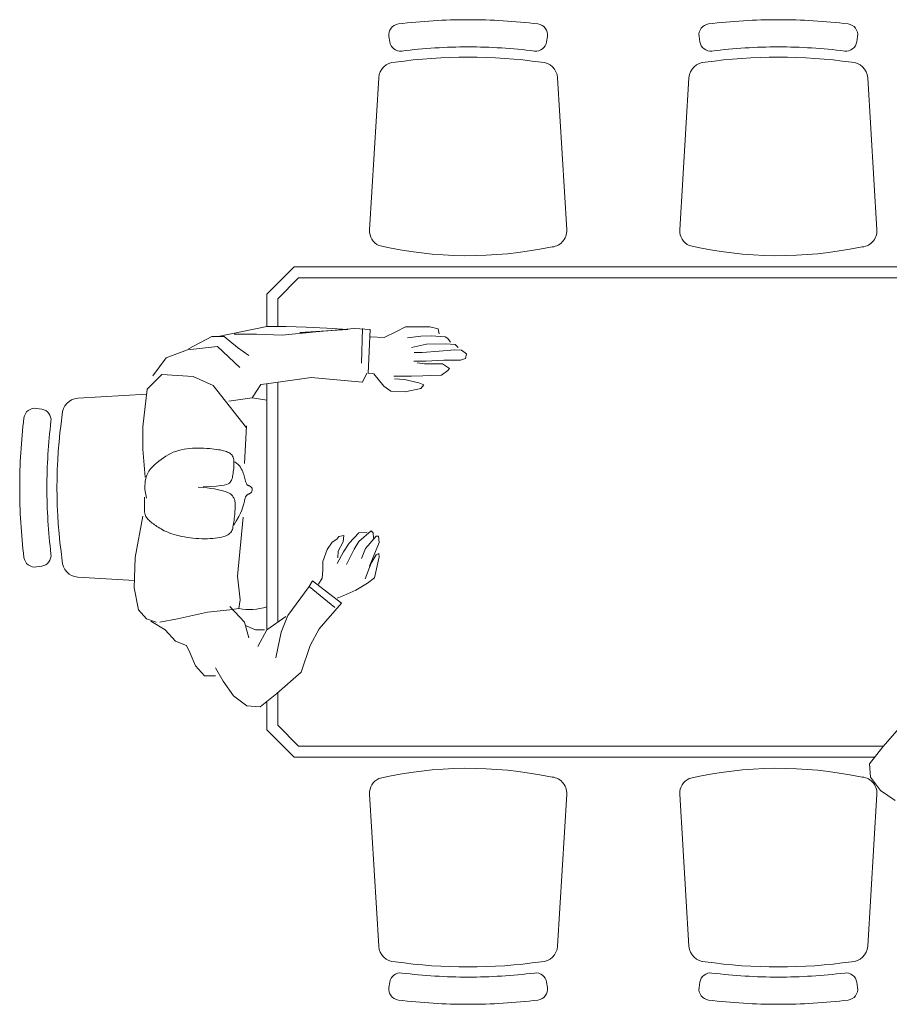
# Model space of a CAD drawing. Units: inches. Extents: x 1913 to 5309, y 1003 to 1733.
# Tile 5 of 23: x 2200 to 2248, y 1415 to 1469. Entities that reach past the tile are written whole.
import ezdxf

# ---------------------------------------------------------------- set-up
doc = ezdxf.new("R2010")
doc.units = ezdxf.units.IN
doc.layers.add('A-FURN', color=8, linetype='Continuous', lineweight=18)

# ---------------------------------------------------------------- blocks, each defined once
blk = doc.blocks.new('A$C421907B3')
for p, q in [((0.7245, 2.5796), (0.7652, 2.5876)), ((0.7652, 2.5876), (0.8209, 2.5856)), ((0.7079, 2.565), (0.7245, 2.5796)), ((0.8209, 2.5856), (0.8965, 2.5714)), ((0.9043, 2.5682), (0.9018, 2.5678)), ((0.9071, 2.5684), (0.9043, 2.5682)), ((0.9102, 2.5686), (0.9071, 2.5684)), ((0.9137, 2.5687), (0.9102, 2.5686)), ((0.9175, 2.5687), (0.9137, 2.5687)), ((0.9217, 2.5687), (0.9175, 2.5687)), ((0.9264, 2.5687), (0.9217, 2.5687)), ((0.9314, 2.5687), (0.9264, 2.5687)), ((0.9684, 2.5672), (1.0195, 2.5715)), ((1.0195, 2.5715), (1.0607, 2.5715)), ((1.0607, 2.5715), (1.1301, 2.5633)), ((0.7038, 2.5568), (0.6875, 2.5302)), ((0.7017, 2.5468), (0.7079, 2.565)), ((0.8808, 2.55), (0.8792, 2.5478)), ((0.8823, 2.5521), (0.8808, 2.55)), ((0.8839, 2.5541), (0.8823, 2.5521)), ((0.8853, 2.556), (0.8839, 2.5541)), ((0.8868, 2.5577), (0.8853, 2.556)), ((0.8883, 2.5594), (0.8868, 2.5577)), ((0.8897, 2.5609), (0.8883, 2.5594)), ((0.8911, 2.5623), (0.8897, 2.5609)), ((0.8926, 2.5635), (0.8911, 2.5623)), ((0.8941, 2.5647), (0.8926, 2.5635)), ((0.8958, 2.5657), (0.8941, 2.5647)), ((0.8976, 2.5665), (0.8958, 2.5657)), ((0.8996, 2.5672), (0.8976, 2.5665)), ((0.9018, 2.5678), (0.8996, 2.5672)), ((0.9361, 2.5662), (0.9297, 2.5647)), ((0.942, 2.5671), (0.9361, 2.5662)), ((0.9475, 2.5676), (0.942, 2.5671)), ((0.9525, 2.5677), (0.9475, 2.5676)), ((0.9571, 2.5675), (0.9525, 2.5677)), ((0.9614, 2.5669), (0.9571, 2.5675)), ((0.9652, 2.5662), (0.9614, 2.5669)), ((0.9686, 2.5653), (0.9652, 2.5662)), ((0.9717, 2.5643), (0.9686, 2.5653)), ((0.9745, 2.5632), (0.9717, 2.5643)), ((0.977, 2.5619), (0.9745, 2.5632)), ((0.9794, 2.5605), (0.977, 2.5619)), ((0.9818, 2.5588), (0.9794, 2.5605)), ((0.9841, 2.5568), (0.9818, 2.5588)), ((0.9865, 2.5545), (0.9841, 2.5568)), ((0.9891, 2.5519), (0.9865, 2.5545)), ((0.9918, 2.5489), (0.9891, 2.5519)), ((1.1301, 2.5633), (1.1567, 2.5368)), ((1.1546, 2.5531), (1.1875, 2.5285)), ((0.7017, 2.5405), (0.7079, 2.5077)), ((0.8699, 2.5321), (0.8684, 2.5289)), ((0.8714, 2.5351), (0.8699, 2.5321)), ((0.873, 2.5379), (0.8714, 2.5351)), ((0.8745, 2.5405), (0.873, 2.5379)), ((0.8761, 2.543), (0.8745, 2.5405)), ((0.8777, 2.5455), (0.8761, 2.543)), ((0.8792, 2.5478), (0.8777, 2.5455)), ((0.9948, 2.5455), (0.9918, 2.5489)), ((0.9978, 2.5419), (0.9948, 2.5455)), ((1.0008, 2.5379), (0.9978, 2.5419)), ((1.0037, 2.5338), (1.0008, 2.5379)), ((1.0066, 2.5294), (1.0037, 2.5338)), ((1.1567, 2.5368), (1.153, 2.4792)), ((0.6875, 2.5302), (0.6672, 2.5117)), ((0.8628, 2.514), (0.8616, 2.5096)), ((0.8641, 2.5181), (0.8628, 2.514)), ((0.8655, 2.522), (0.8641, 2.5181)), ((0.8669, 2.5256), (0.8655, 2.522)), ((0.8684, 2.5289), (0.8669, 2.5256)), ((1.0093, 2.5249), (1.0066, 2.5294)), ((1.0117, 2.5203), (1.0093, 2.5249)), ((1.0138, 2.5155), (1.0117, 2.5203)), ((1.0156, 2.5107), (1.0138, 2.5155)), ((1.1875, 2.5285), (1.202, 2.4895)), ((0.6672, 2.5117), (0.6589, 2.4912)), ((0.7079, 2.5077), (0.7204, 2.4524)), ((0.8594, 2.5001), (0.8584, 2.4951)), ((0.8604, 2.5049), (0.8594, 2.5001)), ((0.8616, 2.5096), (0.8604, 2.5049)), ((1.0171, 2.5058), (1.0156, 2.5107)), ((1.0184, 2.5008), (1.0171, 2.5058)), ((1.0194, 2.4958), (1.0184, 2.5008)), ((1.0202, 2.4907), (1.0194, 2.4958)), ((0.6464, 2.4852), (0.6219, 2.4749)), ((0.6589, 2.4912), (0.6464, 2.4852)), ((0.8562, 2.4794), (0.8558, 2.474)), ((0.8568, 2.4847), (0.8562, 2.4794)), ((0.8576, 2.49), (0.8568, 2.4847)), ((0.8584, 2.4951), (0.8576, 2.49)), ((1.0208, 2.4855), (1.0202, 2.4907)), ((1.0212, 2.4802), (1.0208, 2.4855)), ((1.0214, 2.4749), (1.0212, 2.4802)), ((1.153, 2.4792), (1.1364, 2.4424)), ((1.202, 2.4895), (1.2083, 2.4342)), ((1.2041, 2.4875), (1.2266, 2.4445)), ((0.6219, 2.4749), (0.6036, 2.4584)), ((0.8552, 2.4632), (0.8551, 2.4579)), ((0.8554, 2.4686), (0.8552, 2.4632)), ((0.8558, 2.474), (0.8554, 2.4686)), ((0.9483, 2.453), (0.9491, 2.4609)), ((0.9491, 2.4609), (0.9498, 2.4698)), ((0.9505, 2.4603), (0.9511, 2.447)), ((1.0212, 2.4591), (1.0214, 2.4643)), ((1.0215, 2.4696), (1.0214, 2.4749)), ((1.0214, 2.4643), (1.0215, 2.4696)), ((0.6036, 2.4584), (0.6036, 2.4379)), ((0.7204, 2.4524), (0.7246, 2.4114)), ((0.8551, 2.4579), (0.8552, 2.4527)), ((0.8552, 2.4527), (0.8554, 2.4476)), ((0.8554, 2.4476), (0.8557, 2.4428)), ((0.8557, 2.4428), (0.8561, 2.4383)), ((0.9465, 2.4399), (0.9474, 2.446)), ((0.9474, 2.446), (0.9483, 2.453)), ((0.9511, 2.447), (0.9518, 2.4364)), ((1.0197, 2.4402), (1.0202, 2.4445)), ((1.0202, 2.4445), (1.0206, 2.4492)), ((1.0206, 2.4492), (1.021, 2.4541)), ((1.021, 2.4541), (1.0212, 2.4591)), ((1.1364, 2.4424), (1.0587, 2.3808)), ((1.2266, 2.4445), (1.2266, 2.422)), ((0.5933, 2.4236), (0.5667, 2.4051)), ((0.6178, 2.4379), (0.5933, 2.4236)), ((0.8561, 2.4383), (0.8567, 2.4341)), ((0.8567, 2.4341), (0.8574, 2.4301)), ((0.8574, 2.4301), (0.8582, 2.4265)), ((0.8582, 2.4265), (0.8591, 2.4232)), ((0.9425, 2.4226), (0.9435, 2.426)), ((0.9435, 2.426), (0.9445, 2.43)), ((0.9445, 2.43), (0.9455, 2.4346)), ((0.9455, 2.4346), (0.9465, 2.4399)), ((0.9518, 2.4364), (0.9526, 2.4283)), ((0.9526, 2.4283), (0.9535, 2.4222)), ((1.0168, 2.423), (1.0174, 2.4259)), ((1.0174, 2.4259), (1.0181, 2.429)), ((1.0181, 2.429), (1.0186, 2.4325)), ((1.0186, 2.4325), (1.0192, 2.4362)), ((1.0192, 2.4362), (1.0197, 2.4402)), ((1.2083, 2.4342), (1.1693, 2.3932)), ((1.2447, 2.3435), (1.2266, 2.4332)), ((0.7308, 2.4114), (0.7018, 2.3846)), ((0.7246, 2.4114), (0.7267, 2.3949)), ((0.8591, 2.4232), (0.8601, 2.4202)), ((0.8601, 2.4202), (0.8612, 2.4176)), ((0.8612, 2.4176), (0.8624, 2.4152)), ((0.8624, 2.4152), (0.8637, 2.4132)), ((0.8637, 2.4132), (0.8651, 2.4114)), ((0.8651, 2.4114), (0.8666, 2.41)), ((0.8666, 2.41), (0.8682, 2.4088)), ((0.8682, 2.4088), (0.87, 2.4078)), ((0.87, 2.4078), (0.872, 2.407)), ((0.872, 2.407), (0.8742, 2.4063)), ((0.8742, 2.4063), (0.8767, 2.4058)), ((0.8767, 2.4058), (0.8794, 2.4052)), ((0.8794, 2.4052), (0.8824, 2.4048)), ((0.9315, 2.4052), (0.9329, 2.406)), ((0.9329, 2.406), (0.9341, 2.4069)), ((0.9341, 2.4069), (0.9353, 2.4079)), ((0.9353, 2.4079), (0.9363, 2.409)), ((0.9363, 2.409), (0.9373, 2.4102)), ((0.9373, 2.4102), (0.9382, 2.4116)), ((0.9382, 2.4116), (0.9391, 2.4131)), ((0.9391, 2.4131), (0.9399, 2.415)), ((0.9399, 2.415), (0.9408, 2.4171)), ((0.9408, 2.4171), (0.9416, 2.4196)), ((0.9416, 2.4196), (0.9425, 2.4226)), ((0.9535, 2.4222), (0.9546, 2.4177)), ((0.9546, 2.4177), (0.9558, 2.4146)), ((0.9558, 2.4146), (0.9572, 2.4124)), ((0.9572, 2.4124), (0.9588, 2.4109)), ((0.9588, 2.4109), (0.9606, 2.4096)), ((0.9606, 2.4096), (0.9626, 2.4086)), ((0.9626, 2.4086), (0.9647, 2.4077)), ((0.9647, 2.4077), (0.9671, 2.407)), ((0.9671, 2.407), (0.9696, 2.4064)), ((0.9696, 2.4064), (0.9722, 2.406)), ((0.9722, 2.406), (0.9751, 2.4055)), ((0.9751, 2.4055), (0.9781, 2.4052)), ((0.9781, 2.4052), (0.9812, 2.4048)), ((1.0025, 2.4049), (1.0047, 2.4055)), ((1.0047, 2.4055), (1.0067, 2.4064)), ((1.0067, 2.4064), (1.0085, 2.4075)), ((1.0085, 2.4075), (1.01, 2.4087)), ((1.01, 2.4087), (1.0113, 2.4102)), ((1.0113, 2.4102), (1.0124, 2.4119)), ((1.0124, 2.4119), (1.0135, 2.4137)), ((1.0135, 2.4137), (1.0144, 2.4158)), ((1.0144, 2.4158), (1.0152, 2.418)), ((1.0152, 2.418), (1.016, 2.4204)), ((1.016, 2.4204), (1.0168, 2.423)), ((1.1077, 2.4136), (1.114, 2.3706)), ((1.2266, 2.422), (1.2062, 2.3974)), ((0.5667, 2.4051), (0.5484, 2.3805)), ((0.7267, 2.3949), (0.7429, 2.3929)), ((0.7429, 2.3929), (0.7861, 2.3972)), ((0.7861, 2.3972), (0.8946, 2.387)), ((0.8801, 2.4042), (0.8884, 2.3992)), ((0.8824, 2.4048), (0.8857, 2.4043)), ((0.8857, 2.4043), (0.8891, 2.4039)), ((0.8884, 2.3992), (0.8957, 2.3952)), ((0.8891, 2.4039), (0.8925, 2.4035)), ((0.8925, 2.4035), (0.896, 2.4031)), ((0.8957, 2.3952), (0.9019, 2.3921)), ((0.896, 2.4031), (0.8995, 2.4027)), ((0.8995, 2.4027), (0.9028, 2.4024)), ((0.9019, 2.3921), (0.9073, 2.3897)), ((0.9028, 2.4024), (0.9059, 2.4022)), ((0.9059, 2.4022), (0.9088, 2.4019)), ((0.9073, 2.3897), (0.9119, 2.3881)), ((0.9088, 2.4019), (0.9114, 2.4018)), ((0.9114, 2.4018), (0.9138, 2.4016)), ((0.9119, 2.3881), (0.9157, 2.3869)), ((0.9138, 2.4016), (0.9161, 2.4016)), ((0.9161, 2.4016), (0.9182, 2.4016)), ((0.9182, 2.4016), (0.9201, 2.4017)), ((0.9201, 2.4017), (0.9219, 2.4019)), ((0.9219, 2.4019), (0.9237, 2.4022)), ((0.9237, 2.4022), (0.9254, 2.4026)), ((0.9254, 2.4026), (0.927, 2.4031)), ((0.927, 2.4031), (0.9286, 2.4037)), ((0.9286, 2.4037), (0.9301, 2.4044)), ((0.9301, 2.4044), (0.9315, 2.4052)), ((0.9757, 2.387), (0.9784, 2.388)), ((0.9784, 2.388), (0.9811, 2.3892)), ((0.9811, 2.3892), (0.9837, 2.3905)), ((0.9812, 2.4048), (0.9844, 2.4045)), ((0.9837, 2.3905), (0.9863, 2.3922)), ((0.9844, 2.4045), (0.9877, 2.4043)), ((0.9863, 2.3922), (0.9889, 2.3941)), ((0.9877, 2.4043), (0.9909, 2.4041)), ((0.9889, 2.3941), (0.9915, 2.3965)), ((0.9909, 2.4041), (0.9941, 2.4041)), ((0.9915, 2.3965), (0.994, 2.3993)), ((0.994, 2.3993), (0.9965, 2.4026)), ((0.9941, 2.4041), (0.9971, 2.4042)), ((0.9971, 2.4042), (0.9999, 2.4044)), ((0.9999, 2.4044), (1.0025, 2.4049)), ((1.2062, 2.3974), (1.1917, 2.3769)), ((1.2308, 2.3624), (1.2308, 2.4035)), ((0.5484, 2.3805), (0.5463, 2.356)), ((0.7018, 2.3846), (0.6731, 2.3766)), ((0.6876, 2.3643), (0.6959, 2.3826)), ((0.9157, 2.3869), (0.919, 2.386)), ((0.919, 2.386), (0.9217, 2.3854)), ((0.9217, 2.3854), (0.924, 2.3849)), ((0.924, 2.3849), (0.926, 2.3844)), ((0.926, 2.3844), (0.9277, 2.384)), ((0.9277, 2.384), (0.929, 2.3837)), ((0.929, 2.3837), (0.9302, 2.3833)), ((0.9302, 2.3833), (0.9312, 2.383)), ((0.9312, 2.383), (0.932, 2.3826)), ((0.932, 2.3826), (0.9327, 2.3823)), ((0.9327, 2.3823), (0.9334, 2.3818)), ((0.9334, 2.3818), (0.934, 2.3813)), ((0.934, 2.3813), (0.9346, 2.3808)), ((0.9346, 2.3808), (0.9351, 2.3803)), ((0.9351, 2.3803), (0.9356, 2.3797)), ((0.9356, 2.3797), (0.936, 2.379)), ((0.936, 2.379), (0.9365, 2.3783)), ((0.9365, 2.3783), (0.9369, 2.3776)), ((0.9369, 2.3776), (0.9372, 2.3769)), ((0.9372, 2.3769), (0.9376, 2.3761)), ((0.9376, 2.3761), (0.938, 2.3753)), ((0.938, 2.3753), (0.9384, 2.3746)), ((0.9384, 2.3746), (0.9389, 2.3738)), ((0.9389, 2.3738), (0.9395, 2.3731)), ((0.9395, 2.3731), (0.9401, 2.3725)), ((0.9401, 2.3725), (0.9408, 2.3719)), ((0.9408, 2.3719), (0.9417, 2.3714)), ((0.9417, 2.3714), (0.9426, 2.371)), ((0.9426, 2.371), (0.9437, 2.3707)), ((0.9437, 2.3707), (0.9447, 2.3706)), ((0.9447, 2.3706), (0.9458, 2.3705)), ((0.9458, 2.3705), (0.9468, 2.3706)), ((0.9468, 2.3706), (0.9478, 2.3708)), ((0.9478, 2.3708), (0.9487, 2.3712)), ((0.9487, 2.3712), (0.9494, 2.3717)), ((0.9494, 2.3717), (0.9501, 2.3723)), ((0.9501, 2.3723), (0.9507, 2.3731)), ((0.9507, 2.3731), (0.9512, 2.3739)), ((0.9512, 2.3739), (0.9517, 2.3747)), ((0.9517, 2.3747), (0.9521, 2.3755)), ((0.9521, 2.3755), (0.9524, 2.3764)), ((0.9524, 2.3764), (0.9527, 2.3771)), ((0.9527, 2.3771), (0.953, 2.3778)), ((0.953, 2.3778), (0.9533, 2.3785)), ((0.9533, 2.3785), (0.9536, 2.379)), ((0.9536, 2.379), (0.954, 2.3796)), ((0.954, 2.3796), (0.9546, 2.3801)), ((0.9546, 2.3801), (0.9554, 2.3805)), ((0.9554, 2.3805), (0.9564, 2.381)), ((0.9564, 2.381), (0.9577, 2.3815)), ((0.9577, 2.3815), (0.9593, 2.382)), ((0.9593, 2.382), (0.9611, 2.3826)), ((0.9611, 2.3826), (0.9632, 2.3832)), ((0.9632, 2.3832), (0.9655, 2.3838)), ((0.9655, 2.3838), (0.9679, 2.3845)), ((0.9679, 2.3845), (0.9705, 2.3853)), ((0.9705, 2.3853), (0.9731, 2.3861)), ((0.9731, 2.3861), (0.9757, 2.387)), ((0.9931, 2.3848), (1.0625, 2.3808)), ((1.114, 2.3706), (1.1095, 2.3436)), ((1.114, 2.3706), (1.1385, 2.3544)), ((0.5463, 2.356), (0.5709, 2.3252)), ((0.6569, 2.3601), (0.6876, 2.3438)), ((0.6876, 2.3478), (0.6876, 2.3643)), ((1.1385, 2.3544), (1.1406, 2.3358)), ((1.2287, 2.3154), (1.2308, 2.3624)), ((0.6876, 2.3438), (0.7122, 2.3088)), ((1.1406, 2.3358), (1.151, 2.262)), ((0.5709, 2.3252), (0.6099, 2.2802)), ((0.6835, 2.317), (0.6365, 2.3273)), ((0.7143, 2.3048), (0.6835, 2.317)), ((1.235, 2.2538), (1.2287, 2.3154)), ((0.7674, 2.2656), (0.7143, 2.3048)), ((0.6099, 2.2802), (0.659, 2.2637)), ((0.659, 2.2637), (0.6898, 2.2475)), ((0.7288, 2.2187), (0.7675, 2.2658)), ((0.7675, 2.2658), (0.7779, 2.2598)), ((1.151, 2.262), (1.1428, 2.1677)), ((0.6898, 2.2475), (0.7368, 2.2065)), ((0.7779, 2.2598), (0.7368, 2.2065)), ((0.7716, 2.2487), (0.7827, 2.2421)), ((1.2413, 2.1822), (1.235, 2.2538)), ((0.7827, 2.2421), (0.7969, 2.2406)), ((0.7969, 2.2406), (0.8131, 2.2406)), ((0.8131, 2.2406), (0.8354, 2.2325)), ((0.8354, 2.2325), (0.8487, 2.2236)), ((0.7509, 2.2021), (0.7458, 2.2146)), ((0.8094, 2.2146), (0.8309, 2.2028)), ((0.8324, 2.2124), (0.8198, 2.2132)), ((0.8494, 2.2036), (0.8324, 2.2124)), ((0.8487, 2.2236), (0.8546, 2.2147)), ((0.8546, 2.2147), (0.859, 2.211)), ((0.859, 2.211), (0.8613, 2.2021)), ((0.7606, 2.1798), (0.7509, 2.2021)), ((0.8079, 2.1969), (0.8361, 2.1828)), ((0.8309, 2.2028), (0.8472, 2.1925)), ((0.8472, 2.1925), (0.8658, 2.1747)), ((0.8613, 2.2021), (0.8494, 2.2036)), ((0.7732, 2.1583), (0.7606, 2.1798)), ((0.8361, 2.1828), (0.8502, 2.1747)), ((0.8502, 2.1747), (0.8695, 2.1518)), ((0.8658, 2.1747), (0.8672, 2.1591)), ((1.2392, 2.1535), (1.2413, 2.1822)), ((0.7835, 2.1457), (0.7732, 2.1583)), ((0.7814, 2.1628), (0.8102, 2.1517)), ((0.848, 2.1369), (0.805, 2.1547)), ((0.8191, 2.1695), (0.8369, 2.1621)), ((0.8369, 2.1621), (0.8599, 2.1429)), ((1.1428, 2.1677), (1.159, 2.1597)), ((1.1595, 2.1573), (1.158, 2.1467)), ((1.1595, 2.1573), (1.2392, 2.1535)), ((1.1777, 2.1697), (1.2413, 2.1677)), ((1.226, 2.1528), (1.2245, 2.1279)), ((0.8221, 2.1369), (0.7835, 2.1457)), ((0.8102, 2.1517), (0.8257, 2.1428)), ((0.828, 2.1376), (0.8221, 2.1369)), ((0.8257, 2.1428), (0.828, 2.1376)), ((0.8599, 2.1384), (0.848, 2.1369)), ((0.8658, 2.1481), (0.8561, 2.1473)), ((0.8599, 2.1429), (0.8599, 2.1384)), ((0.8695, 2.1518), (0.8658, 2.1481)), ((1.158, 2.1467), (1.1354, 2.1286)), ((1.1354, 2.1286), (1.1263, 2.1158)), ((1.2245, 2.1279), (1.2358, 2.1052)), ((1.1263, 2.1158), (1.1248, 2.0893)), ((1.1474, 2.0909), (1.149, 2.1089)), ((1.1535, 2.1105), (1.1536, 2.078)), ((1.2358, 2.1052), (1.2442, 2.0886)), ((1.1248, 2.0893), (1.1308, 2.0606)), ((1.1414, 2.0644), (1.1474, 2.0909)), ((1.2238, 2.0848), (1.2269, 2.0606)), ((1.2442, 2.0886), (1.2442, 2.0441)), ((1.1377, 2.0553), (1.1414, 2.0644)), ((1.1536, 2.078), (1.1543, 2.0568)), ((1.1762, 2.0539), (1.1784, 2.0674)), ((1.1815, 2.0735), (1.1815, 2.0516)), ((1.1974, 2.0584), (1.1974, 2.0727)), ((1.2064, 2.078), (1.2125, 2.0501)), ((1.1308, 2.0606), (1.1377, 2.0553)), ((1.1543, 2.0568), (1.1551, 2.0432)), ((1.1762, 2.0357), (1.1762, 2.0539)), ((1.1815, 2.0516), (1.1831, 2.0183)), ((1.1996, 2.0267), (1.1974, 2.0584)), ((1.2125, 2.0501), (1.2132, 2.0154)), ((1.2269, 2.0606), (1.2276, 2.0418)), ((1.2442, 2.0441), (1.2404, 2.029)), ((1.1551, 2.0432), (1.1558, 2.0229)), ((1.1762, 2.0206), (1.1762, 2.0357)), ((1.2019, 1.9979), (1.1996, 2.0267)), ((1.2276, 2.0418), (1.2261, 2.0161)), ((1.2404, 2.029), (1.2314, 2.0267)), ((1.1558, 2.0229), (1.1641, 2.0108)), ((1.1641, 2.0108), (1.168, 2.0077)), ((1.168, 2.0077), (1.1762, 2.0206)), ((1.1831, 2.0183), (1.1831, 1.9874)), ((1.2132, 2.0154), (1.2117, 1.9972)), ((1.223, 2.0108), (1.2163, 2.0063)), ((1.2261, 2.0161), (1.223, 2.0108)), ((1.2012, 1.9859), (1.2019, 1.9979)), ((1.2117, 1.9972), (1.2064, 1.9919)), ((1.1831, 1.9874), (1.186, 1.9783)), ((1.186, 1.9783), (1.1944, 1.9768)), ((1.1944, 1.9768), (1.2012, 1.9859)), ((0.3928, 1.2157), (0.4173, 1.234)), ((0.4173, 1.234), (0.4418, 1.2361)), ((0.4418, 1.2361), (0.4726, 1.2115)), ((0.3742, 1.1891), (0.3928, 1.2157)), ((0.4726, 1.2115), (0.5176, 1.1724))]:
    blk.add_line(p, q)
at = {"ltscale": 0.1}
for points in [[(0.9489, 2.7478, 0.030867), (0.827, 2.7403, -0.408428), (0.8047, 2.7573), (0.8033, 2.7672, -0.419966), (0.8206, 2.7899, -0.030916), (0.9489, 2.7978, -0.030916), (1.0772, 2.7899, -0.419966), (1.0945, 2.7672), (1.0931, 2.7573, -0.408428), (1.0708, 2.7403, 0.030867)], [(0.0782, 2.1079, -0.399285), (0.1067, 2.1378), (0.3861, 2.1548, -0.305593), (0.4148, 2.1375, -0.109362), (0.4176, 1.8225, -0.429301), (0.3861, 1.7925), (0.1067, 1.8094, -0.399285), (0.0782, 1.8394, -0.071734)], [(1.7302, 2.1079, 0.399285), (1.7017, 2.1378), (1.4223, 2.1548, 0.305593), (1.3936, 2.1375, 0.109362), (1.3908, 1.8225, 0.429301), (1.4223, 1.7925), (1.7017, 1.8094, 0.399285), (1.7302, 1.8394, 0.071734)], [(0.05, 1.9736, 0.030867), (0.0575, 1.8517, -0.408428), (0.0405, 1.8294), (0.0306, 1.828, -0.419966), (0.0079, 1.8453, -0.030916), (0, 1.9736, -0.030916), (0.0079, 2.1019, -0.419966), (0.0306, 2.1193), (0.0405, 2.1178, -0.408428), (0.0575, 2.0956, 0.030867)], [(1.7584, 1.9736, -0.030867), (1.7509, 1.8517, 0.408428), (1.7679, 1.8294), (1.7778, 1.828, 0.419966), (1.8005, 1.8453, 0.030916), (1.8084, 1.9736, 0.030916), (1.8005, 2.1019, 0.419966), (1.7778, 2.1193), (1.7679, 2.1178, 0.408428), (1.7509, 2.0956, -0.030867)], [(0.0782, 1.5378, -0.399285), (0.1067, 1.5678), (0.3861, 1.5847, -0.305593), (0.4148, 1.5674, -0.109362), (0.4176, 1.2524, -0.429301), (0.3861, 1.2224), (0.1067, 1.2393, -0.399285), (0.0782, 1.2693, -0.071734)], [(1.7302, 1.5378, 0.399285), (1.7017, 1.5678), (1.4223, 1.5847, 0.305593), (1.3936, 1.5674, 0.109362), (1.3908, 1.2524, 0.429301), (1.4223, 1.2224), (1.7017, 1.2393, 0.399285), (1.7302, 1.2693, 0.071734)], [(0.05, 1.4036, 0.030867), (0.0575, 1.2816, -0.408428), (0.0405, 1.2593), (0.0306, 1.2579, -0.419966), (0.0079, 1.2752, -0.030916), (0, 1.4036, -0.030916), (0.0079, 1.5319, -0.419966), (0.0306, 1.5492), (0.0405, 1.5478, -0.408428), (0.0575, 1.5255, 0.030867)], [(1.7584, 1.4036, -0.030867), (1.7509, 1.2816, 0.408428), (1.7679, 1.2593), (1.7778, 1.2579, 0.419966), (1.8005, 1.2752, 0.030916), (1.8084, 1.4036, 0.030916), (1.8005, 1.5319, 0.419966), (1.7778, 1.5492), (1.7679, 1.5478, 0.408428), (1.7509, 1.5255, -0.030867)]]:
    blk.add_lwpolyline(points, format="xyb", close=True, dxfattribs=at)
blk.add_lwpolyline([(0.7784, 2.5871), (0.7847, 2.6911, -0.399285), (0.8147, 2.7196, -0.071734), (1.0831, 2.7196, -0.399285), (1.1131, 2.6911), (1.1208, 2.5644)], format="xyb", dxfattribs=at)
for points in [[(0.4542, 1.2262), (0.4542, 2.2936), (0.5042, 2.3436), (0.5562, 2.3436)], [(0.6878, 2.3436), (1.1397, 2.3436)], [(1.2446, 2.3436), (1.3042, 2.3436), (1.3542, 2.2936), (1.3542, 1.0533)], [(0.4742, 1.2101), (0.4742, 2.2853), (0.5125, 2.3236), (0.5723, 2.3236)], [(0.7018, 2.3236), (1.1423, 2.3236)], [(1.245, 2.3234), (1.2959, 2.3236), (1.3342, 2.2853), (1.3342, 1.0419)]]:
    blk.add_lwpolyline(points, dxfattribs=at)
blk.add_lwpolyline([(1.2332, 2.2712), (1.2341, 2.2831), (1.2396, 2.1946), (1.2396, 2.1946), (1.2419, 2.2332), (1.2437, 2.2711), (1.2448, 2.3081), (1.2452, 2.3436)])
blk.add_arc((0.8297, 2.3756), 0.1048, 169.4107, 197.7809)

msp = doc.modelspace()

# ---------------------------------------------------------------- block references
at = {"layer": 'A-FURN', "xscale": 30.26057373645948, "yscale": 30.26057373645948, "zscale": 30.26057373645948, "rotation": 89.99999999999996}
msp.add_blockref('A$C421907B3', (2284.376, 1414.678), dxfattribs=at)

doc.saveas('drawing.dxf')
